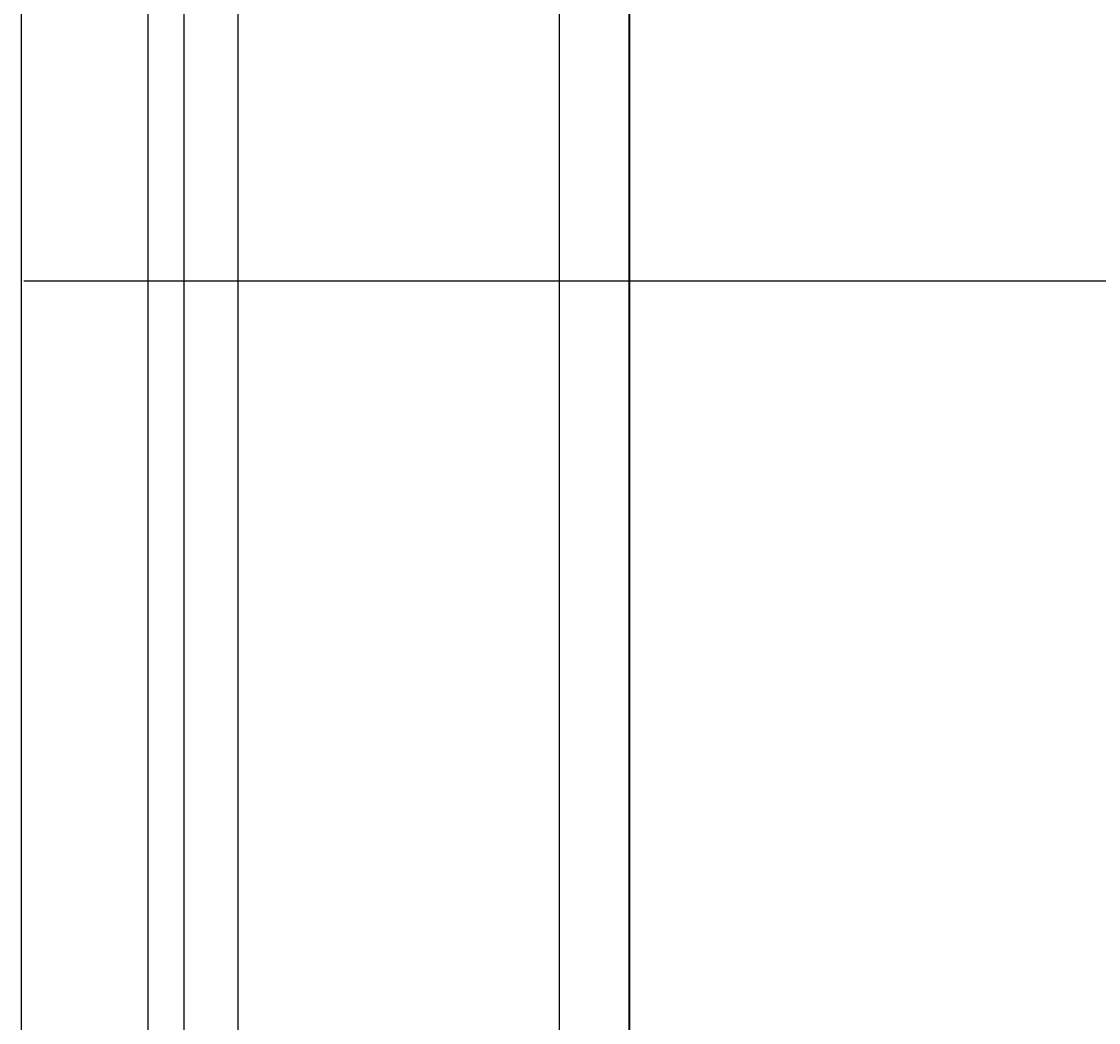
# Model space of a CAD drawing. Units: inches. Extents: x -6 to 289, y -8 to 323.
# Tile 40 of 107: x 230 to 260, y 96 to 124. Entities that reach past the tile are written whole.
import ezdxf

# ---------------------------------------------------------------- set-up
doc = ezdxf.new("R2010")
doc.units = ezdxf.units.IN
doc.header["$MEASUREMENT"] = 0
doc.layers.add('A-ANNO-DIMS', color=2, linetype='Continuous', lineweight=18)
doc.layers.add('A-ELEV', color=7, linetype='Continuous', lineweight=35)
doc.styles.get("Standard").update_dxf_attribs({"font": 'arial.ttf'})
doc.dimstyles.get("Standard").update_dxf_attribs({"dimtxt": 0.18, "dimasz": 0.18, "dimexe": 0.18, "dimexo": 0.0625, "dimgap": 0.09, "dimtad": 0, "dimtih": 1, "dimtoh": 1, "dimdec": 4, "dimzin": 0, "dimdsep": 46, "dimtxsty": 'Standard', "dimcen": 0.09, "dimadec": 0, "dimazin": 0, "dimtfac": 1, "dimtdec": 4, "dimtofl": 0, "dimtmove": 0, "dimatfit": 3, "dimfxl": 1, "dimtolj": 1, "dimtzin": 0, "dimarcsym": 0})

# ---------------------------------------------------------------- blocks, each defined once
blk = doc.blocks.new('*D15')
at = {"layer": 'A-ANNO-DIMS', "color": 0, "lineweight": -2, "transparency": 16777216}
for p, q in [((247.164, 162.411), (247.164, 322.969)), ((247.344, 322.789), (258.944, 322.789)), ((270.984, 322.789), (259.384, 322.789)), ((271.164, 7.351), (271.164, 322.969))]:
    blk.add_line(p, q, dxfattribs=at)
at = {"layer": 'A-ANNO-DIMS', "color": 0, "transparency": 16777216}
for points in [[(247.344, 322.819), (247.344, 322.759), (247.164, 322.789)], [(270.984, 322.819), (270.984, 322.759), (271.164, 322.789)]]:
    blk.add_solid(points, dxfattribs=at)
at = {"layer": 'Defpoints', "color": 0, "transparency": 16777216}
for p in [(271.164, 322.789), (247.164, 162.348), (271.164, 7.289)]:
    blk.add_point(p, dxfattribs=at)
at = {"layer": 'A-ANNO-DIMS', "color": 0, "transparency": 16777216, "insert": (259.164, 322.789), "char_height": 0.18, "attachment_point": 5}
blk.add_mtext('\\A1;24', dxfattribs=at)
blk = doc.blocks.new('*D23')
at = {"layer": 'A-ANNO-DIMS', "color": 0, "lineweight": -2, "transparency": 16777216}
for p, q in [((259.226, 127.289), (288.653, 127.289)), ((288.473, 127.109), (288.473, 67.471)), ((288.473, 7.469), (288.473, 67.107)), ((271.226, 7.289), (288.653, 7.289))]:
    blk.add_line(p, q, dxfattribs=at)
at = {"layer": 'A-ANNO-DIMS', "color": 0, "transparency": 16777216}
for points in [[(288.443, 127.109), (288.503, 127.109), (288.473, 127.289)], [(288.443, 7.469), (288.503, 7.469), (288.473, 7.289)]]:
    blk.add_solid(points, dxfattribs=at)
at = {"layer": 'Defpoints', "color": 0, "transparency": 16777216}
for p in [(259.164, 127.289), (288.473, 127.289), (271.164, 7.289)]:
    blk.add_point(p, dxfattribs=at)
at = {"layer": 'A-ANNO-DIMS', "color": 0, "transparency": 16777216, "insert": (288.473, 67.289), "char_height": 0.18, "attachment_point": 5}
blk.add_mtext('\\A1;120', dxfattribs=at)
blk = doc.blocks.new('*D44')
at = {"layer": 'A-ANNO-DIMS', "color": 0, "lineweight": -2, "transparency": 16777216}
for p, q in [((212.292, 224.326), (212.292, -8.391)), ((233.792, 224.326), (233.792, -8.391)), ((212.472, -8.211), (222.716, -8.211)), ((233.612, -8.211), (223.368, -8.211))]:
    blk.add_line(p, q, dxfattribs=at)
at = {"layer": 'A-ANNO-DIMS', "color": 0, "transparency": 16777216}
for points in [[(212.472, -8.181), (212.472, -8.241), (212.292, -8.211)], [(233.612, -8.181), (233.612, -8.241), (233.792, -8.211)]]:
    blk.add_solid(points, dxfattribs=at)
at = {"layer": 'Defpoints', "color": 0, "transparency": 16777216}
for p in [(212.292, 224.389), (233.792, 224.389), (233.792, -8.211)]:
    blk.add_point(p, dxfattribs=at)
at = {"layer": 'A-ANNO-DIMS', "color": 0, "transparency": 16777216, "insert": (223.042, -8.211), "char_height": 0.18, "attachment_point": 5}
blk.add_mtext('\\A1;21.5', dxfattribs=at)
blk = doc.blocks.new('*D45')
at = {"layer": 'A-ANNO-DIMS', "color": 0, "lineweight": -2, "transparency": 16777216}
for p, q in [((234.792, 225.326), (234.792, -8.391)), ((233.792, 224.326), (233.792, -8.391)), ((233.972, -8.211), (234.169, -8.211)), ((234.612, -8.211), (234.415, -8.211))]:
    blk.add_line(p, q, dxfattribs=at)
at = {"layer": 'A-ANNO-DIMS', "color": 0, "transparency": 16777216}
for points in [[(233.972, -8.181), (233.972, -8.241), (233.792, -8.211)], [(234.612, -8.181), (234.612, -8.241), (234.792, -8.211)]]:
    blk.add_solid(points, dxfattribs=at)
at = {"layer": 'Defpoints', "color": 0, "transparency": 16777216}
for p in [(234.792, 225.389), (233.792, 224.389), (234.792, -8.211)]:
    blk.add_point(p, dxfattribs=at)
at = {"layer": 'A-ANNO-DIMS', "color": 0, "transparency": 16777216, "insert": (234.292, -8.211), "char_height": 0.18, "attachment_point": 5}
blk.add_mtext('\\A1;1', dxfattribs=at)
blk = doc.blocks.new('*D46')
at = {"layer": 'A-ANNO-DIMS', "color": 0, "lineweight": -2, "transparency": 16777216}
for p, q in [((236.292, 226.826), (236.292, -8.391)), ((234.792, 225.326), (234.792, -8.391)), ((234.972, -8.211), (235.296, -8.211)), ((236.112, -8.211), (235.788, -8.211))]:
    blk.add_line(p, q, dxfattribs=at)
at = {"layer": 'A-ANNO-DIMS', "color": 0, "transparency": 16777216}
for points in [[(234.972, -8.181), (234.972, -8.241), (234.792, -8.211)], [(236.112, -8.181), (236.112, -8.241), (236.292, -8.211)]]:
    blk.add_solid(points, dxfattribs=at)
at = {"layer": 'Defpoints', "color": 0, "transparency": 16777216}
for p in [(236.292, 226.889), (234.792, 225.389), (236.292, -8.211)]:
    blk.add_point(p, dxfattribs=at)
at = {"layer": 'A-ANNO-DIMS', "color": 0, "transparency": 16777216, "insert": (235.542, -8.211), "char_height": 0.18, "attachment_point": 5}
blk.add_mtext('\\A1;1.5', dxfattribs=at)
blk = doc.blocks.new('*D80')
at = {"layer": 'A-ANNO-DIMS', "color": 0, "lineweight": -2, "transparency": 16777216}
for p, q in [((188.292, 116.842), (188.292, 322.969)), ((188.472, 322.789), (209.07, 322.789)), ((230.112, 322.789), (209.513, 322.789)), ((230.292, 116.842), (230.292, 322.969))]:
    blk.add_line(p, q, dxfattribs=at)
at = {"layer": 'A-ANNO-DIMS', "color": 0, "transparency": 16777216}
for points in [[(188.472, 322.819), (188.472, 322.759), (188.292, 322.789)], [(230.112, 322.819), (230.112, 322.759), (230.292, 322.789)]]:
    blk.add_solid(points, dxfattribs=at)
at = {"layer": 'Defpoints', "color": 0, "transparency": 16777216}
for p in [(230.292, 322.789), (188.292, 116.779), (230.292, 116.779)]:
    blk.add_point(p, dxfattribs=at)
at = {"layer": 'A-ANNO-DIMS', "color": 0, "transparency": 16777216, "insert": (209.292, 322.789), "char_height": 0.18, "attachment_point": 5}
blk.add_mtext('\\A1;42', dxfattribs=at)
blk = doc.blocks.new('*D81')
at = {"layer": 'A-ANNO-DIMS', "color": 0, "lineweight": -2, "transparency": 16777216}
for p, q in [((230.292, 68.842), (230.292, 322.969)), ((230.472, 322.789), (237.298, 322.789)), ((245.035, 322.789), (238.208, 322.789)), ((245.215, 66.286), (245.215, 322.969))]:
    blk.add_line(p, q, dxfattribs=at)
at = {"layer": 'A-ANNO-DIMS', "color": 0, "transparency": 16777216}
for points in [[(230.472, 322.819), (230.472, 322.759), (230.292, 322.789)], [(245.035, 322.819), (245.035, 322.759), (245.215, 322.789)]]:
    blk.add_solid(points, dxfattribs=at)
at = {"layer": 'Defpoints', "color": 0, "transparency": 16777216}
for p in [(245.215, 322.789), (230.292, 68.779), (245.215, 66.224)]:
    blk.add_point(p, dxfattribs=at)
at = {"layer": 'A-ANNO-DIMS', "color": 0, "transparency": 16777216, "insert": (237.753, 322.789), "char_height": 0.18, "attachment_point": 5}
blk.add_mtext('\\A1;14.923', dxfattribs=at)
blk = doc.blocks.new('*D82')
at = {"layer": 'A-ANNO-DIMS', "color": 0, "lineweight": -2, "transparency": 16777216}
for p, q in [((245.215, 66.286), (245.215, 322.969)), ((245.395, 322.789), (258.699, 322.789)), ((272.793, 322.789), (259.489, 322.789)), ((272.973, 66.286), (272.973, 322.969))]:
    blk.add_line(p, q, dxfattribs=at)
at = {"layer": 'A-ANNO-DIMS', "color": 0, "transparency": 16777216}
for points in [[(245.395, 322.819), (245.395, 322.759), (245.215, 322.789)], [(272.793, 322.819), (272.793, 322.759), (272.973, 322.789)]]:
    blk.add_solid(points, dxfattribs=at)
at = {"layer": 'Defpoints', "color": 0, "transparency": 16777216}
for p in [(272.973, 322.789), (245.215, 66.224), (272.973, 66.224)]:
    blk.add_point(p, dxfattribs=at)
at = {"layer": 'A-ANNO-DIMS', "color": 0, "transparency": 16777216, "insert": (259.094, 322.789), "char_height": 0.18, "attachment_point": 5}
blk.add_mtext('\\A1;27.76', dxfattribs=at)
blk = doc.blocks.new('*D91')
at = {"layer": 'A-ANNO-DIMS', "color": 0, "lineweight": -2, "transparency": 16777216}
for p, q in [((230.354, 116.779), (288.653, 116.779)), ((288.473, 116.599), (288.473, 92.961)), ((288.473, 68.959), (288.473, 92.598)), ((230.354, 68.779), (288.653, 68.779))]:
    blk.add_line(p, q, dxfattribs=at)
at = {"layer": 'A-ANNO-DIMS', "color": 0, "transparency": 16777216}
for points in [[(288.443, 116.599), (288.503, 116.599), (288.473, 116.779)], [(288.443, 68.959), (288.503, 68.959), (288.473, 68.779)]]:
    blk.add_solid(points, dxfattribs=at)
at = {"layer": 'Defpoints', "color": 0, "transparency": 16777216}
for p in [(230.292, 116.779), (288.473, 116.779), (230.292, 68.779)]:
    blk.add_point(p, dxfattribs=at)
at = {"layer": 'A-ANNO-DIMS', "color": 0, "transparency": 16777216, "insert": (288.473, 92.779), "char_height": 0.18, "attachment_point": 5}
blk.add_mtext('\\A1;48', dxfattribs=at)

msp = doc.modelspace()

# ---------------------------------------------------------------- linework, layer by layer
at = {"layer": 'A-ELEV'}
msp.add_line((247.1638, 68.4323), (247.1638, 127.2888), dxfattribs=at)

# ---------------------------------------------------------------- dimensions: what is measured, and where the dimension line sits
at = {"layer": 'A-ANNO-DIMS'}
for base, p1, p2, override, picture, middle in [((230.2918, 322.7888), (188.2918, 116.7795), (230.2918, 116.7795), {"dimdec": 0, "dimlfac": 1, "dimrnd": 0, "dimzin": 0, "dimdsep": 46, "dimlunit": 2}, '*D80', (209.2918, 322.7888)), ((245.2146, 322.7888), (230.2918, 68.7795), (245.2146, 66.2238), {"dimdec": 3, "dimlfac": 1, "dimrnd": 0, "dimzin": 0, "dimdsep": 46, "dimlunit": 2}, '*D81', (237.7532, 322.7888)), ((272.9733, 322.7888), (245.2146, 66.2238), (272.9733, 66.2238), {"dimdec": 2, "dimlfac": 1, "dimrnd": 0, "dimzin": 0, "dimdsep": 46, "dimlunit": 2}, '*D82', (259.0939, 322.7888)), ((271.1638, 322.7888), (247.1638, 162.3484), (271.1638, 7.2888), {"dimdec": 0, "dimlfac": 1, "dimrnd": 0, "dimzin": 0, "dimdsep": 46, "dimlunit": 2}, '*D15', (259.1638, 322.7888)), ((236.2918, -8.2112), (234.7918, 225.3887), (236.2918, 226.8887), {"dimdec": 1, "dimlfac": 1, "dimrnd": 0, "dimzin": 0, "dimdsep": 46, "dimlunit": 2}, '*D46', (235.5418, -8.2112)), ((234.7918, -8.2112), (233.7918, 224.3887), (234.7918, 225.3887), {"dimdec": 0, "dimlfac": 1, "dimrnd": 0, "dimzin": 0, "dimdsep": 46, "dimlunit": 2}, '*D45', (234.2918, -8.2112)), ((233.7918, -8.2112), (212.2918, 224.3887), (233.7918, 224.3887), {"dimdec": 1, "dimlfac": 1, "dimrnd": 0, "dimzin": 0, "dimdsep": 46, "dimlunit": 2}, '*D44', (223.0418, -8.2112))]:
    dim = msp.add_linear_dim(base=base, p1=p1, p2=p2, dimstyle='Standard', override=override, dxfattribs=at)
    dim.commit()
    dim.dimension.update_dxf_attribs({"geometry": picture, "text_midpoint": middle})
for base, p1, p2, picture, middle in [((288.4733, 127.2888), (271.1638, 7.2888), (259.1638, 127.2888), '*D23', (288.4733, 67.2888)), ((288.4733, 116.7795), (230.2918, 68.7795), (230.2918, 116.7795), '*D91', (288.4733, 92.7795))]:
    dim = msp.add_linear_dim(base=base, p1=p1, p2=p2, angle=90, dimstyle='Standard', override={"dimdec": 0, "dimlfac": 1, "dimrnd": 0, "dimzin": 0, "dimdsep": 46, "dimlunit": 2}, dxfattribs=at)
    dim.commit()
    dim.dimension.update_dxf_attribs({"geometry": picture, "text_midpoint": middle})

doc.saveas('drawing.dxf')
